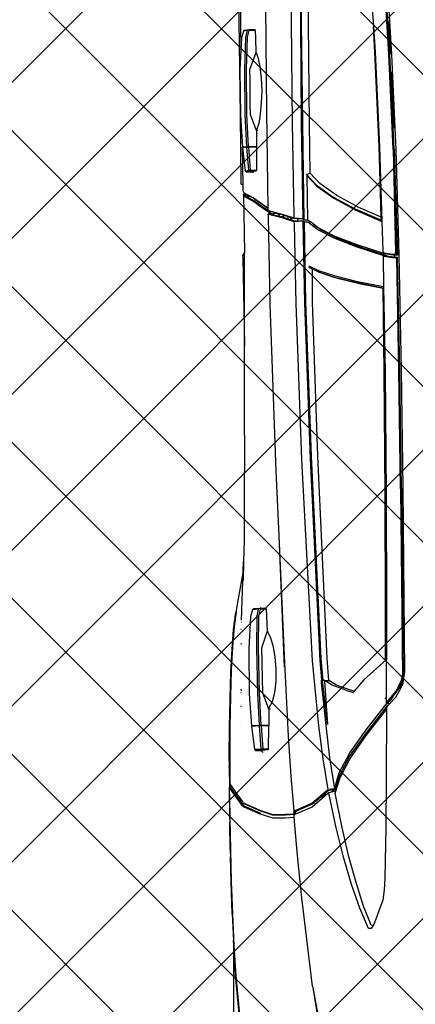
# Model space of a CAD drawing. Units: inches. Extents: x 2167 to 2589, y 1680 to 2489.
# Tile 15 of 38: x 2335 to 2353, y 1727 to 1772. Entities that reach past the tile are written whole.
import ezdxf

# ---------------------------------------------------------------- set-up
doc = ezdxf.new("R2010")
doc.units = ezdxf.units.IN
doc.header["$MEASUREMENT"] = 0
doc.layers.get('0').update_dxf_attribs({"color": 250})
doc.layers.add('C-PRKG-VEHS', color=8, linetype='Continuous', lineweight=13)
doc.layers.add('L-PVMT-PATT', color=252, linetype='Continuous', lineweight=13)
doc.layers.add('Edges', color=250, linetype='Continuous')

# ---------------------------------------------------------------- blocks, each defined once
blk = doc.blocks.new('Nissan Qashqai pl')
at = {"layer": 'Edges'}
for p, q in [((9.6953, 11.2892), (9.863, 11.2944)), ((9.6954, 11.2907), (9.8641, 11.2959)), ((9.696, 11.2932), (9.8644, 11.2982)), ((9.7669, 11.2945), (9.7832, 11.2951)), ((9.8629, 11.2925), (9.863, 11.2944)), ((9.8641, 11.2959), (9.863, 11.2944)), ((9.8638, 11.2934), (9.8641, 11.2959)), ((9.8644, 11.2982), (10.0472, 11.3018)), ((9.8681, 11.2959), (9.8678, 11.2935)), ((10.0476, 11.2996), (9.8681, 11.2959)), ((9.8681, 11.2959), (9.869, 11.2946)), ((9.869, 11.2946), (9.8689, 11.2927)), ((10.0477, 11.2982), (9.869, 11.2946)), ((10.0472, 11.3018), (10.2357, 11.3043)), ((10.2367, 11.3022), (10.0476, 11.2996)), ((10.2369, 11.3008), (10.0477, 11.2982)), ((10.2357, 11.3043), (10.53, 11.3068)), ((10.2367, 11.3022), (10.5351, 11.305)), ((10.2369, 11.3008), (10.5348, 11.3036)), ((10.4153, 11.3058), (10.2954, 11.3046)), ((10.4153, 11.3058), (10.4174, 11.3058)), ((10.4174, 11.3058), (10.4181, 11.3058)), ((10.4181, 11.3058), (10.4182, 11.3058)), ((10.4182, 11.3058), (10.53, 11.3068)), ((10.53, 11.3068), (10.5301, 11.3068)), ((10.5301, 11.3068), (10.5323, 11.3065)), ((10.5323, 11.3065), (10.5419, 11.3051)), ((10.5422, 11.3021), (10.5348, 11.3036)), ((10.5424, 11.3035), (10.5351, 11.305)), ((10.5366, 11.3048), (10.536, 11.305)), ((10.5379, 11.3052), (10.5381, 11.305)), ((10.5419, 11.3051), (10.5463, 11.3031)), ((10.5419, 11.3051), (10.5479, 11.3042)), ((10.5522, 11.2977), (10.5422, 11.3021)), ((10.5472, 11.3014), (10.5424, 11.3035)), ((10.5463, 11.3031), (10.5551, 11.2984)), ((10.5546, 11.2982), (10.5472, 11.3014)), ((10.5479, 11.3042), (10.5589, 11.2991)), ((10.5598, 11.2935), (10.5522, 11.2977)), ((10.5583, 11.296), (10.5546, 11.2982)), ((10.5551, 11.2984), (10.5583, 11.296)), ((10.5612, 11.2944), (10.5583, 11.296)), ((10.5589, 11.2991), (10.57, 11.2925)), ((10.5683, 11.2885), (10.5612, 11.2944)), ((9.5437, 11.2822), (9.4735, 11.2779)), ((9.5438, 11.2836), (9.4736, 11.2793)), ((9.4739, 11.282), (9.5443, 11.2863)), ((9.491, 11.2819), (9.5434, 11.2852)), ((9.6953, 11.2892), (9.5437, 11.2822)), ((9.6954, 11.2907), (9.5438, 11.2836)), ((9.5443, 11.2863), (9.696, 11.2932)), ((9.5717, 11.2865), (9.6618, 11.2907)), ((9.6953, 11.2892), (9.8598, 11.2925)), ((9.8652, 11.2788), (9.8516, 11.2363)), ((9.8629, 11.2925), (9.8598, 11.2925)), ((9.8605, 11.2746), (9.8626, 11.2878)), ((9.8615, 11.2754), (9.8635, 11.2886)), ((9.8626, 11.2878), (9.8627, 11.2909)), ((9.8627, 11.2909), (9.8629, 11.2925)), ((9.8627, 11.2909), (9.8637, 11.291)), ((9.8635, 11.2886), (9.8637, 11.291)), ((9.8637, 11.291), (9.8638, 11.2934)), ((9.8637, 11.291), (9.8643, 11.291)), ((9.8643, 11.291), (9.8677, 11.291)), ((9.8652, 11.2738), (9.8652, 11.2788)), ((9.8675, 11.2887), (9.8655, 11.2754)), ((9.8686, 11.2879), (9.8665, 11.2747)), ((9.8677, 11.291), (9.8675, 11.2887)), ((9.8678, 11.2935), (9.8677, 11.291)), ((9.8689, 11.2927), (9.8686, 11.2879)), ((10.2453, 11.2777), (10.4289, 11.2783)), ((10.4289, 11.2783), (10.5092, 11.2783)), ((10.5099, 11.2768), (10.5092, 11.2783)), ((10.5092, 11.2783), (10.5094, 11.2783)), ((10.5094, 11.2783), (10.51, 11.2776)), ((10.5783, 11.2783), (10.5094, 11.2783)), ((10.5764, 11.28), (10.5598, 11.2935)), ((10.5683, 11.2885), (10.573, 11.285)), ((10.575, 11.2829), (10.5683, 11.2885)), ((10.57, 11.2925), (10.5811, 11.2822)), ((10.573, 11.285), (10.5769, 11.2818)), ((10.5776, 11.2808), (10.575, 11.2829)), ((10.5783, 11.2783), (10.5764, 11.28)), ((10.5796, 11.2787), (10.5776, 11.2808)), ((10.5776, 11.2808), (10.5783, 11.2783)), ((10.5796, 11.2787), (10.5783, 11.2783)), ((10.5796, 11.2824), (10.5796, 11.2787)), ((10.6215, 11.2456), (10.5796, 11.2787)), ((10.5811, 11.2822), (10.5821, 11.2808)), ((10.5811, 11.2822), (10.5834, 11.28)), ((10.5821, 11.2808), (10.5834, 11.2793)), ((10.5825, 11.2806), (10.5834, 11.2793)), ((10.5834, 11.28), (10.5851, 11.2783)), ((10.5834, 11.2793), (10.5835, 11.2793)), ((10.5835, 11.2793), (10.584, 11.2787)), ((10.584, 11.2789), (10.584, 11.2793)), ((10.584, 11.2787), (10.584, 11.2789)), ((10.584, 11.2787), (10.6261, 11.2458)), ((10.584, 11.2787), (10.5851, 11.2783)), ((10.5843, 11.2787), (10.584, 11.2787)), ((10.5847, 11.2787), (10.5843, 11.2787)), ((10.5851, 11.2783), (10.5892, 11.2783)), ((10.6306, 11.2459), (10.5892, 11.2783)), ((10.5892, 11.2783), (10.6988, 11.2779)), ((10.6988, 11.2779), (10.7769, 11.2774)), ((9.5403, 11.26), (9.6913, 11.2674)), ((9.6912, 11.2667), (9.5404, 11.2598)), ((9.8039, 11.27), (9.6912, 11.2667)), ((9.6913, 11.2674), (9.8099, 11.2711)), ((9.8039, 11.27), (9.7884, 11.2343)), ((9.7905, 11.2283), (9.8087, 11.2702)), ((9.7925, 11.2294), (9.8107, 11.2711)), ((9.8087, 11.2702), (9.8039, 11.27)), ((9.8099, 11.2711), (9.8087, 11.2702)), ((9.8099, 11.2711), (9.8107, 11.2711)), ((9.8107, 11.2711), (9.8573, 11.2726)), ((9.8475, 11.2312), (9.8611, 11.2734)), ((9.8652, 11.2738), (9.8516, 11.2313)), ((9.8573, 11.2726), (9.8603, 11.2727)), ((9.8603, 11.2727), (9.8605, 11.2746)), ((9.8611, 11.2734), (9.8603, 11.2727)), ((9.8612, 11.2735), (9.8611, 11.2734)), ((9.8612, 11.2735), (9.8615, 11.2754)), ((9.8655, 11.2754), (9.8652, 11.2738)), ((9.8652, 11.2735), (9.8665, 11.2747)), ((9.8652, 11.2738), (9.8652, 11.2738)), ((9.8652, 11.2738), (9.8652, 11.2735)), ((9.8652, 11.2735), (9.8664, 11.2728)), ((9.8665, 11.2747), (9.8664, 11.2728)), ((9.8664, 11.2728), (9.9149, 11.2736)), ((9.9149, 11.2736), (9.9066, 11.2322)), ((9.9169, 11.2728), (9.9086, 11.2313)), ((9.9177, 11.2728), (9.9106, 11.2373)), ((9.9149, 11.2736), (10.0505, 11.276)), ((9.9177, 11.2728), (9.9169, 11.2728)), ((10.0501, 11.2747), (9.9177, 11.2728)), ((10.2453, 11.2762), (10.0501, 11.2747)), ((10.0505, 11.276), (10.2453, 11.2777)), ((10.4292, 11.2767), (10.2453, 11.2762)), ((10.5099, 11.2768), (10.4292, 11.2767)), ((10.51, 11.2776), (10.5099, 11.2768)), ((10.51, 11.2776), (10.5419, 11.2423)), ((10.5705, 11.2771), (10.5709, 11.2767)), ((10.5709, 11.2767), (10.5719, 11.2759)), ((10.7769, 11.2774), (10.858, 11.2759)), ((10.858, 11.2759), (10.8766, 11.2745)), ((10.8766, 11.2745), (10.8932, 11.2722)), ((10.8932, 11.2722), (10.932, 11.258)), ((9.471, 11.2554), (9.4997, 11.2573)), ((9.4997, 11.2573), (9.5403, 11.26)), ((9.5404, 11.2598), (9.4997, 11.2573)), ((10.933, 11.2541), (10.9026, 11.2417)), ((10.9384, 11.2497), (10.9059, 11.2355)), ((10.932, 11.258), (10.9335, 11.257)), ((10.9335, 11.257), (10.933, 11.2541)), ((10.9335, 11.257), (10.9386, 11.2537)), ((10.9386, 11.2537), (10.9384, 11.2497)), ((9.7884, 11.2343), (9.7692, 11.1989)), ((9.8338, 11.1956), (9.8475, 11.2312)), ((9.8516, 11.2363), (9.8378, 11.2007)), ((9.8516, 11.2313), (9.8378, 11.1957)), ((9.9066, 11.2322), (9.8978, 11.197)), ((9.9086, 11.2313), (9.8998, 11.196)), ((9.9106, 11.2373), (9.9018, 11.2021)), ((10.5419, 11.2423), (10.56, 11.2265)), ((10.6583, 11.2197), (10.6215, 11.2456)), ((10.6261, 11.2458), (10.6627, 11.22)), ((10.6671, 11.2203), (10.6306, 11.2459)), ((10.9026, 11.2417), (10.8653, 11.2297)), ((10.9059, 11.2355), (10.8682, 11.2226)), ((9.7713, 11.1929), (9.7905, 11.2283)), ((9.7733, 11.194), (9.7925, 11.2294)), ((10.5584, 11.2206), (10.5502, 11.1986)), ((10.56, 11.2265), (10.5584, 11.2206)), ((10.5584, 11.2136), (10.5617, 11.2251)), ((10.56, 11.2265), (10.5617, 11.2251)), ((10.69, 11.2028), (10.6583, 11.2197)), ((10.6627, 11.22), (10.6943, 11.2032)), ((10.6976, 11.2041), (10.6671, 11.2203)), ((10.8239, 11.2181), (10.7754, 11.2071)), ((10.8653, 11.2297), (10.8239, 11.2181)), ((10.8682, 11.2226), (10.8264, 11.21)), ((9.8378, 11.2007), (9.8241, 11.1736)), ((9.9018, 11.2021), (9.8931, 11.1752)), ((10.5584, 11.2136), (10.5502, 11.1916)), ((10.7155, 11.1952), (10.69, 11.2028)), ((10.6943, 11.2032), (10.7155, 11.1969)), ((10.7228, 11.1965), (10.6976, 11.2041)), ((10.7754, 11.2071), (10.7228, 11.1965)), ((10.8264, 11.21), (10.7776, 11.1982)), ((9.7692, 11.1989), (9.7499, 11.1721)), ((9.7519, 11.1661), (9.7713, 11.1929)), ((9.754, 11.1672), (9.7733, 11.194)), ((9.8201, 11.1685), (9.8338, 11.1956)), ((9.8378, 11.1957), (9.8241, 11.1686)), ((9.8978, 11.197), (9.8891, 11.1701)), ((9.8911, 11.1693), (9.8998, 11.196)), ((10.543, 11.1865), (10.5079, 11.1835)), ((10.5502, 11.1986), (10.543, 11.1865)), ((10.5502, 11.1916), (10.543, 11.1795)), ((10.543, 11.1795), (10.543, 11.1865)), ((10.5439, 11.1796), (10.613, 11.1841)), ((10.613, 11.1841), (10.547, 11.1767)), ((10.6144, 11.1813), (10.6664, 11.1875)), ((10.6664, 11.1875), (10.7155, 11.1952)), ((10.7137, 11.1846), (10.6678, 11.177)), ((10.7165, 11.1851), (10.7137, 11.1846)), ((10.7155, 11.1957), (10.7155, 11.1969)), ((10.7155, 11.1969), (10.7192, 11.1957)), ((10.7209, 11.1902), (10.7155, 11.1957)), ((10.7155, 11.1952), (10.7155, 11.1957)), ((10.7186, 11.1848), (10.7155, 11.1952)), ((10.7155, 11.1952), (10.7165, 11.1851)), ((10.7177, 11.1838), (10.7165, 11.1851)), ((10.7387, 11.1593), (10.7177, 11.1838)), ((10.7312, 11.1701), (10.7186, 11.1848)), ((10.7192, 11.1957), (10.7228, 11.1965)), ((10.7192, 11.1957), (10.7209, 11.1902)), ((10.7209, 11.1902), (10.7221, 11.1861)), ((10.7221, 11.1861), (10.7222, 11.1859)), ((10.7222, 11.186), (10.7221, 11.1861)), ((10.7247, 11.1867), (10.7222, 11.186)), ((10.7222, 11.186), (10.7222, 11.1859)), ((10.7222, 11.1859), (10.7232, 11.1848)), ((10.7222, 11.1859), (10.7224, 11.1855)), ((10.7224, 11.1855), (10.7312, 11.1701)), ((10.7232, 11.1848), (10.7228, 11.1859)), ((10.7232, 11.1848), (10.7449, 11.1598)), ((10.7776, 11.1982), (10.7247, 11.1867)), ((10.7257, 11.1853), (10.7256, 11.1854)), ((11.0357, 11.1613), (11.1598, 11.1847)), ((9.7499, 11.1721), (9.7337, 11.1566)), ((9.8241, 11.1686), (9.8119, 11.1529)), ((9.8241, 11.1736), (9.8147, 11.1616)), ((9.8147, 11.1616), (9.8201, 11.1685)), ((9.8891, 11.1701), (9.8818, 11.1551)), ((9.8911, 11.1691), (9.8867, 11.16)), ((9.8931, 11.1751), (9.8911, 11.1693)), ((9.8911, 11.1693), (9.8911, 11.1691)), ((9.8931, 11.1751), (9.8931, 11.1752)), ((10.1849, 11.1687), (9.9393, 11.1602)), ((10.5079, 11.1835), (10.1849, 11.1687)), ((10.5079, 11.1739), (10.1849, 11.1585)), ((10.1894, 11.1563), (10.5109, 11.1721)), ((10.543, 11.1771), (10.5079, 11.1739)), ((10.5109, 11.1721), (10.5417, 11.1748)), ((10.6152, 11.1702), (10.5113, 11.1603)), ((10.543, 11.1771), (10.5417, 11.1748)), ((10.5417, 11.1748), (10.5427, 11.1739)), ((10.5436, 11.1754), (10.5427, 11.1739)), ((10.5427, 11.1739), (10.5458, 11.1742)), ((10.5439, 11.1796), (10.543, 11.1795)), ((10.543, 11.1795), (10.543, 11.1771)), ((10.544, 11.1763), (10.543, 11.1771)), ((10.544, 11.1763), (10.5436, 11.1754)), ((10.547, 11.1767), (10.544, 11.1763)), ((10.5458, 11.1742), (10.6144, 11.1813)), ((10.6678, 11.177), (10.6152, 11.1702)), ((10.7397, 11.1602), (10.7312, 11.1701)), ((11.0492, 11.1635), (11.1336, 11.1772)), ((9.4936, 11.1538), (9.3225, 11.1531)), ((9.6552, 11.1554), (9.4936, 11.1538)), ((9.7337, 11.1566), (9.6552, 11.1554)), ((9.7357, 11.1507), (9.7337, 11.1566)), ((9.7357, 11.1507), (9.7519, 11.1661)), ((9.7378, 11.1517), (9.754, 11.1672)), ((9.8078, 11.1528), (9.7378, 11.1517)), ((9.8078, 11.1528), (9.8119, 11.1579)), ((9.8078, 11.1471), (9.8078, 11.1528)), ((9.8147, 11.1616), (9.8119, 11.1579)), ((9.8119, 11.1579), (9.8119, 11.1529)), ((9.8119, 11.1529), (9.8119, 11.1472)), ((9.8147, 11.1616), (9.8147, 11.1616)), ((9.8867, 11.16), (9.8838, 11.1541)), ((9.9393, 11.1602), (9.8867, 11.16)), ((10.1849, 11.1585), (9.9393, 11.1497)), ((9.9411, 11.1475), (10.1894, 11.1563)), ((10.5113, 11.1603), (10.19, 11.1433)), ((10.7501, 11.1327), (10.7387, 11.1593)), ((10.7507, 11.1344), (10.7397, 11.1602)), ((10.7449, 11.1598), (10.7563, 11.1333)), ((11.0304, 11.1603), (10.8896, 11.1434)), ((11.0304, 11.1603), (11.0357, 11.1613)), ((11.0357, 11.1613), (11.0491, 11.1635)), ((11.0492, 11.1635), (11.0491, 11.1635)), ((9.3198, 11.1403), (9.4922, 11.1409)), ((9.4936, 11.1428), (9.3225, 11.1421)), ((9.4922, 11.1409), (9.654, 11.1423)), ((9.6552, 11.1445), (9.4936, 11.1428)), ((9.654, 11.1423), (9.8061, 11.1447)), ((9.8078, 11.1471), (9.6552, 11.1445)), ((9.7357, 11.1507), (9.7378, 11.1517)), ((9.8061, 11.1447), (9.8051, 11.1309)), ((9.8055, 11.1298), (9.8058, 11.1369)), ((9.8058, 11.1369), (9.8061, 11.1447)), ((9.8098, 11.1369), (9.8058, 11.1369)), ((9.8061, 11.1447), (9.8078, 11.1471)), ((9.8098, 11.1369), (9.8096, 11.13)), ((9.8101, 11.1449), (9.8098, 11.1369)), ((9.8101, 11.1449), (9.9411, 11.1475)), ((9.8119, 11.1472), (9.8101, 11.1449)), ((9.8101, 11.1449), (9.8112, 11.1311)), ((9.9393, 11.1497), (9.8119, 11.1472)), ((10.19, 11.1433), (9.9414, 11.1341)), ((10.8218, 11.1365), (10.7615, 11.1311)), ((10.8896, 11.1434), (10.8218, 11.1365)), ((9.4919, 11.1269), (9.3194, 11.1262)), ((9.6538, 11.1284), (9.4919, 11.1269)), ((9.802, 11.1309), (9.6538, 11.1284)), ((9.7992, 11.1133), (9.8044, 11.129)), ((9.803, 11.1212), (9.8014, 11.1176)), ((9.8014, 11.1176), (9.8026, 11.1212)), ((9.8051, 11.1309), (9.802, 11.1309)), ((9.8026, 11.1212), (9.8041, 11.1256)), ((9.803, 11.1212), (9.8026, 11.1212)), ((9.8067, 11.1213), (9.803, 11.1212)), ((9.8041, 11.1256), (9.8045, 11.1268)), ((9.8041, 11.1256), (9.8081, 11.1256)), ((9.8044, 11.129), (9.8051, 11.1309)), ((9.8067, 11.1213), (9.8044, 11.1142)), ((9.8045, 11.1268), (9.8046, 11.1271)), ((9.8045, 11.1268), (9.8085, 11.1268)), ((9.8046, 11.1271), (9.8055, 11.1298)), ((9.8086, 11.1271), (9.8046, 11.1271)), ((9.8106, 11.1292), (9.8054, 11.1135)), ((9.8081, 11.1256), (9.8067, 11.1213)), ((9.8085, 11.1268), (9.8081, 11.1256)), ((9.8086, 11.1271), (9.8085, 11.1268)), ((9.8096, 11.13), (9.8086, 11.1271)), ((9.8112, 11.1311), (9.8106, 11.1292)), ((9.8143, 11.1312), (9.8112, 11.1311)), ((9.9414, 11.1341), (9.8143, 11.1312)), ((10.5147, 11.1156), (10.6318, 11.1213)), ((10.6318, 11.1213), (10.6955, 11.1257)), ((10.6955, 11.1257), (10.7509, 11.1302)), ((10.7507, 11.1309), (10.7501, 11.1327)), ((10.7511, 11.1335), (10.7507, 11.1344)), ((10.7507, 11.1344), (10.7524, 11.1335)), ((10.751, 11.131), (10.7507, 11.1309)), ((10.7509, 11.1302), (10.7507, 11.1309)), ((10.7522, 11.1311), (10.7509, 11.1302)), ((10.7516, 11.131), (10.7509, 11.1302)), ((10.7519, 11.1314), (10.7511, 11.1335)), ((10.7519, 11.1314), (10.7516, 11.131)), ((10.7522, 11.1311), (10.7516, 11.131)), ((10.7526, 11.1318), (10.7519, 11.1314)), ((10.7553, 11.1307), (10.7522, 11.1311)), ((10.7524, 11.1335), (10.7526, 11.1318)), ((10.7524, 11.1335), (10.7556, 11.1319)), ((10.7532, 11.1321), (10.7526, 11.1318)), ((10.7526, 11.1318), (10.7526, 11.1314)), ((10.7556, 11.1319), (10.7532, 11.1321)), ((10.7563, 11.1169), (10.7553, 11.1307)), ((10.7556, 11.1319), (10.7561, 11.1317)), ((10.7563, 11.1319), (10.7561, 11.1319)), ((10.7563, 11.1315), (10.7561, 11.1317)), ((10.7561, 11.1317), (10.7563, 11.1317)), ((10.7563, 11.1333), (10.7569, 11.1317)), ((10.7563, 11.1317), (10.7563, 11.1319)), ((10.7563, 11.1317), (10.7569, 11.1317)), ((10.7569, 11.1316), (10.7563, 11.1317)), ((10.7563, 11.1315), (10.7563, 11.1317)), ((10.7572, 11.1178), (10.7563, 11.1315)), ((10.7573, 11.1307), (10.7563, 11.1315)), ((10.7569, 11.1317), (10.7569, 11.1316)), ((10.7569, 11.1316), (10.7573, 11.1307)), ((10.7604, 11.131), (10.7573, 11.1307)), ((10.7615, 11.1311), (10.7604, 11.131)), ((10.7615, 11.1311), (10.7623, 11.1173)), ((9.7937, 11.0918), (9.7992, 11.1133)), ((9.7987, 11.1053), (9.7977, 11.1033)), ((9.7978, 11.1044), (9.7987, 11.108)), ((9.7987, 11.1053), (9.7978, 11.1044)), ((9.7987, 11.108), (9.8002, 11.1141)), ((9.7992, 11.1065), (9.7987, 11.108)), ((9.7992, 11.1065), (9.7987, 11.1053)), ((9.8027, 11.1078), (9.7992, 11.1065)), ((9.8054, 11.1135), (9.7999, 11.0919)), ((9.8002, 11.1141), (9.8008, 11.1157)), ((9.8027, 11.1078), (9.8003, 11.0983)), ((9.8008, 11.1157), (9.8014, 11.1176)), ((9.8014, 11.1139), (9.8008, 11.1157)), ((9.8043, 11.1139), (9.8014, 11.1139)), ((9.8031, 11.1093), (9.8014, 11.1139)), ((9.8031, 11.1093), (9.8027, 11.1078)), ((9.8043, 11.1139), (9.8031, 11.1093)), ((9.8044, 11.1142), (9.8043, 11.1139)), ((10.2081, 11.1017), (10.312, 11.1064)), ((10.312, 11.1064), (10.5147, 11.1156)), ((10.312, 11.1064), (10.5214, 11.1149)), ((10.7565, 11.0969), (10.7563, 11.1169)), ((10.7575, 11.0979), (10.7572, 11.1178)), ((10.7623, 11.1173), (10.7626, 11.0974)), ((9.7965, 11.0915), (9.7894, 11.0806)), ((9.7931, 11.089), (9.7934, 11.0906)), ((9.7933, 11.0892), (9.7941, 11.0901)), ((9.7934, 11.0906), (9.7937, 11.0918)), ((9.7934, 11.0906), (9.7938, 11.0904)), ((9.7941, 11.0901), (9.7943, 11.0907)), ((9.7964, 11.0988), (9.7943, 11.0907)), ((9.7955, 11.0925), (9.7943, 11.0907)), ((9.7963, 11.0918), (9.7955, 11.0925)), ((9.7992, 11.0966), (9.7963, 11.0918)), ((9.7963, 11.0918), (9.7963, 11.0918)), ((9.7964, 11.0917), (9.7963, 11.0918)), ((9.7964, 11.0988), (9.7973, 11.1023)), ((9.7964, 11.0988), (9.7992, 11.0966)), ((9.7964, 11.0917), (9.7996, 11.0966)), ((9.7964, 11.0917), (9.7964, 11.0917)), ((9.7967, 11.0915), (9.7964, 11.0917)), ((9.7965, 11.0915), (9.7967, 11.0915)), ((9.7983, 11.0901), (9.7965, 11.0915)), ((9.7967, 11.0915), (9.7986, 11.0916)), ((9.7977, 11.0907), (9.7967, 11.0915)), ((9.7973, 11.1023), (9.7977, 11.1042)), ((9.7977, 11.1033), (9.7973, 11.1023)), ((9.7973, 11.1023), (9.7977, 11.1011)), ((9.7977, 11.1042), (9.7978, 11.1044)), ((9.7977, 11.1042), (9.7977, 11.1033)), ((9.7977, 11.1011), (9.7977, 11.0998)), ((9.7977, 11.1011), (9.7985, 11.099)), ((9.7977, 11.0998), (9.7985, 11.099)), ((9.7982, 11.0902), (9.7977, 11.0907)), ((9.7986, 11.0916), (9.7982, 11.0902)), ((9.7983, 11.0901), (9.7982, 11.0902)), ((9.7986, 11.0898), (9.7983, 11.0901)), ((9.7985, 11.099), (9.7989, 11.098)), ((9.7988, 11.0925), (9.7986, 11.0916)), ((9.7986, 11.0898), (9.7993, 11.0891)), ((9.7998, 11.0964), (9.7988, 11.0925)), ((9.7989, 11.098), (9.7998, 11.0976)), ((9.7998, 11.0976), (9.7992, 11.0966)), ((9.7999, 11.0919), (9.7993, 11.0891)), ((9.8002, 11.098), (9.7996, 11.0966)), ((9.8001, 11.0974), (9.7996, 11.0966)), ((9.7996, 11.0966), (9.7998, 11.0964)), ((9.8003, 11.0983), (9.7998, 11.0976)), ((9.8001, 11.0974), (9.7998, 11.0964)), ((9.8002, 11.098), (9.8001, 11.0974)), ((9.8003, 11.0983), (9.8002, 11.098)), ((9.8024, 11.0892), (9.9426, 11.0923)), ((9.9426, 11.0923), (10.2081, 11.1017)), ((10.4653, 11.0881), (10.4652, 11.0897)), ((10.4653, 11.0881), (10.4732, 11.0925)), ((10.4732, 11.0925), (10.4871, 11.0967)), ((10.4871, 11.0967), (10.5048, 11.1002)), ((10.5048, 11.1002), (10.5246, 11.1019)), ((10.5246, 11.1019), (10.5445, 11.1017)), ((10.5445, 11.1017), (10.5625, 11.0996)), ((10.5625, 11.0996), (10.5769, 11.0957)), ((10.5867, 11.0897), (10.563, 11.0809)), ((10.5769, 11.0957), (10.5863, 11.0904)), ((10.5863, 11.0904), (10.5867, 11.0897)), ((10.5885, 11.0904), (10.5867, 11.0897)), ((10.5885, 11.0931), (10.5885, 11.0904)), ((10.5885, 11.0904), (10.6141, 11.0905)), ((10.6141, 11.0905), (10.615, 11.0905)), ((10.6142, 11.0782), (10.6141, 11.0905)), ((10.6517, 11.0902), (10.615, 11.0905)), ((10.615, 11.0905), (10.6151, 11.0782)), ((10.6518, 11.0808), (10.6517, 11.0902)), ((10.6517, 11.0902), (10.6535, 11.0895)), ((10.6535, 11.0895), (10.6543, 11.0786)), ((10.6535, 11.0895), (10.6536, 11.0803)), ((10.7497, 11.0763), (10.7565, 11.0969)), ((10.7507, 11.0773), (10.7575, 11.0979)), ((10.7626, 11.0974), (10.7559, 11.0767)), ((9.4673, 11.0852), (9.6358, 11.0866)), ((9.5503, 11.0736), (9.5641, 11.076)), ((9.5641, 11.076), (9.5818, 11.0782)), ((9.5818, 11.0782), (9.6016, 11.0791)), ((9.6016, 11.0791), (9.6215, 11.0782)), ((9.6215, 11.0782), (9.6395, 11.0766)), ((9.6358, 11.0866), (9.7887, 11.0889)), ((9.6395, 11.0766), (9.654, 11.0744)), ((9.654, 11.0744), (9.6633, 11.0715)), ((9.7728, 11.066), (9.7832, 11.0805)), ((9.7738, 11.067), (9.7842, 11.0814)), ((9.7883, 11.0815), (9.7778, 11.0671)), ((9.7894, 11.0806), (9.7788, 11.0661)), ((9.7832, 11.0805), (9.7887, 11.0889)), ((9.7842, 11.0814), (9.7891, 11.0889)), ((9.7933, 11.0892), (9.7883, 11.0815)), ((9.7887, 11.0889), (9.7891, 11.0889)), ((9.7891, 11.0889), (9.79, 11.0889)), ((9.79, 11.0889), (9.7931, 11.089)), ((9.7931, 11.089), (9.7933, 11.0892)), ((9.7993, 11.0891), (9.8024, 11.0892)), ((10.4263, 11.0777), (10.4274, 11.0767)), ((10.4274, 11.0767), (10.4275, 11.0856)), ((10.4274, 11.0762), (10.4274, 11.0767)), ((10.4282, 11.0666), (10.4274, 11.0762)), ((10.4275, 11.0856), (10.4293, 11.0863)), ((10.4293, 11.0863), (10.4291, 11.0765)), ((10.4291, 11.0765), (10.4398, 11.0741)), ((10.4398, 11.0718), (10.4291, 11.0741)), ((10.4291, 11.0741), (10.4299, 11.0644)), ((10.4293, 11.0863), (10.4398, 11.0868)), ((10.4398, 11.0868), (10.4653, 11.0878)), ((10.4398, 11.0741), (10.4909, 11.0734)), ((10.4653, 11.0877), (10.4653, 11.0881)), ((10.4653, 11.0878), (10.4653, 11.0881)), ((10.4653, 11.0881), (10.4653, 11.0881)), ((10.4653, 11.0877), (10.4653, 11.0878)), ((10.4908, 11.0793), (10.4653, 11.0877)), ((10.563, 11.0809), (10.4908, 11.0793)), ((10.4909, 11.0734), (10.563, 11.075)), ((10.563, 11.075), (10.6142, 11.0779)), ((10.6142, 11.0756), (10.5631, 11.0727)), ((10.6142, 11.0779), (10.6142, 11.0782)), ((10.6142, 11.0765), (10.6142, 11.0779)), ((10.615, 11.0765), (10.6142, 11.0765)), ((10.6142, 11.0756), (10.6142, 11.0765)), ((10.615, 11.0639), (10.6142, 11.0756)), ((10.6151, 11.0765), (10.615, 11.0765)), ((10.615, 11.0765), (10.6151, 11.0639)), ((10.6151, 11.078), (10.6518, 11.0808)), ((10.6518, 11.0784), (10.6151, 11.0756)), ((10.6151, 11.0782), (10.6151, 11.078)), ((10.6151, 11.078), (10.6151, 11.0765)), ((10.6151, 11.0765), (10.6151, 11.0756)), ((10.6151, 11.0756), (10.616, 11.0629)), ((10.6518, 11.0784), (10.6518, 11.0808)), ((10.6518, 11.0808), (10.6536, 11.0803)), ((10.6536, 11.0803), (10.6518, 11.0784)), ((10.6526, 11.0674), (10.6518, 11.0784)), ((10.6536, 11.0803), (10.6537, 11.0783)), ((10.6543, 11.0786), (10.6537, 11.0783)), ((10.6537, 11.0783), (10.6543, 11.0693)), ((10.6578, 11.0814), (10.6543, 11.0786)), ((10.6543, 11.0693), (10.6543, 11.0786)), ((10.7385, 11.051), (10.7497, 11.0763)), ((10.7396, 11.0519), (10.7507, 11.0773)), ((10.7549, 11.0776), (10.743, 11.0503)), ((10.7559, 11.0767), (10.7448, 11.0511)), ((9.5037, 11.0635), (9.5045, 11.0628)), ((9.5044, 11.0586), (9.5045, 11.0628)), ((9.5052, 11.0524), (9.5044, 11.0586)), ((9.5045, 11.0683), (9.5063, 11.0687)), ((9.5045, 11.0628), (9.5045, 11.0683)), ((9.5063, 11.0687), (9.5061, 11.0586)), ((9.5061, 11.0586), (9.5167, 11.0559)), ((9.5063, 11.0687), (9.5168, 11.0691)), ((9.5168, 11.0691), (9.5423, 11.0696)), ((9.5422, 11.0706), (9.5422, 11.0716)), ((9.5422, 11.0706), (9.5424, 11.0707)), ((9.5423, 11.0696), (9.5422, 11.0706)), ((9.5426, 11.0695), (9.5423, 11.0696)), ((9.5424, 11.0707), (9.5503, 11.0736)), ((9.5426, 11.0695), (9.5424, 11.0707)), ((9.5667, 11.0609), (9.5426, 11.0695)), ((9.5678, 11.0604), (9.5667, 11.0609)), ((9.5846, 11.0606), (9.5678, 11.0604)), ((9.6236, 11.0609), (9.5846, 11.0606)), ((9.64, 11.0611), (9.6236, 11.0609)), ((9.6413, 11.0616), (9.64, 11.0611)), ((9.6645, 11.0705), (9.6413, 11.0616)), ((9.6633, 11.0715), (9.6645, 11.0705)), ((9.6655, 11.0708), (9.6645, 11.0705)), ((9.6655, 11.0728), (9.6655, 11.0708)), ((9.6655, 11.0708), (9.6911, 11.0709)), ((9.6911, 11.0709), (9.692, 11.0709)), ((9.6911, 11.0645), (9.6911, 11.0709)), ((9.6912, 11.0631), (9.6911, 11.0645)), ((9.692, 11.0631), (9.6912, 11.0631)), ((9.6912, 11.0577), (9.6912, 11.0631)), ((9.692, 11.0709), (9.692, 11.0645)), ((9.692, 11.0709), (9.7287, 11.0708)), ((9.692, 11.0645), (9.692, 11.0631)), ((9.692, 11.0631), (9.6921, 11.0578)), ((9.6921, 11.0578), (9.7288, 11.0609)), ((9.7288, 11.0588), (9.6922, 11.0556)), ((9.7287, 11.0708), (9.7305, 11.0704)), ((9.7288, 11.0609), (9.7287, 11.0708)), ((9.7288, 11.0588), (9.7288, 11.0609)), ((9.7288, 11.0609), (9.7306, 11.0607)), ((9.7306, 11.0607), (9.7288, 11.0588)), ((9.7296, 11.0527), (9.7288, 11.0588)), ((9.7305, 11.0704), (9.7313, 11.0644)), ((9.7305, 11.0704), (9.7306, 11.0607)), ((9.7306, 11.0607), (9.7314, 11.0547)), ((9.733, 11.066), (9.7313, 11.0644)), ((9.7314, 11.0547), (9.7313, 11.0644)), ((9.7674, 11.0557), (9.7728, 11.066)), ((9.7684, 11.0567), (9.7717, 11.0631)), ((9.7717, 11.0631), (9.7707, 11.0593)), ((9.7707, 11.0593), (9.7709, 11.0549)), ((9.7717, 11.0631), (9.7738, 11.067)), ((9.7778, 11.0671), (9.7724, 11.0568)), ((9.7788, 11.0661), (9.7734, 11.0558)), ((10.4282, 11.0666), (10.4299, 11.0644)), ((10.4299, 11.0644), (10.4406, 11.0612)), ((10.4909, 11.0711), (10.4398, 11.0718)), ((10.4406, 11.0612), (10.4919, 11.0584)), ((10.5631, 11.0727), (10.4909, 11.0711)), ((10.4919, 11.0584), (10.564, 11.0591)), ((10.564, 11.0591), (10.6151, 11.0628)), ((10.6151, 11.0639), (10.615, 11.0639)), ((10.6151, 11.0628), (10.615, 11.0639)), ((10.6151, 11.0639), (10.6151, 11.0628)), ((10.616, 11.0629), (10.6526, 11.0674)), ((10.6526, 11.0674), (10.6543, 11.0693)), ((9.2517, 11.0411), (9.5372, 11.0459)), ((9.641, 11.045), (9.351, 11.0411)), ((9.5052, 11.0524), (9.5069, 11.0501)), ((9.5168, 11.0537), (9.5061, 11.0564)), ((9.5061, 11.0564), (9.5069, 11.0501)), ((9.5069, 11.0501), (9.5176, 11.0469)), ((9.5167, 11.0559), (9.5679, 11.0543)), ((9.5679, 11.0521), (9.5168, 11.0537)), ((9.5176, 11.0469), (9.5372, 11.0459)), ((9.5372, 11.0459), (9.5689, 11.0442)), ((9.5679, 11.0543), (9.64, 11.0549)), ((9.6401, 11.0528), (9.5679, 11.0521)), ((9.5689, 11.0442), (9.641, 11.045)), ((9.64, 11.0549), (9.6912, 11.0577)), ((9.6913, 11.0556), (9.6401, 11.0528)), ((9.641, 11.045), (9.6921, 11.0485)), ((9.7466, 11.0464), (9.641, 11.045)), ((9.6913, 11.0556), (9.6912, 11.0577)), ((9.692, 11.0499), (9.6913, 11.0556)), ((9.6922, 11.0499), (9.692, 11.0499)), ((9.6921, 11.0485), (9.692, 11.0499)), ((9.6922, 11.0556), (9.6921, 11.0578)), ((9.6922, 11.0499), (9.6921, 11.0485)), ((9.7526, 11.0495), (9.6921, 11.0485)), ((9.6922, 11.0556), (9.693, 11.0486)), ((9.6922, 11.0556), (9.6922, 11.0499)), ((9.693, 11.0486), (9.7296, 11.0527)), ((9.7296, 11.0527), (9.7314, 11.0547)), ((9.7511, 11.0463), (9.7466, 11.0464)), ((9.7526, 11.0495), (9.7511, 11.0463)), ((9.7623, 11.0497), (9.7526, 11.0495)), ((9.7623, 11.0497), (9.7643, 11.0504)), ((9.7643, 11.0504), (9.7652, 11.0514)), ((9.7643, 11.0504), (9.7648, 11.0513)), ((9.7648, 11.0513), (9.7664, 11.054)), ((9.7648, 11.0513), (9.7648, 11.0513)), ((9.7652, 11.0514), (9.7665, 11.0535)), ((9.7664, 11.054), (9.7674, 11.0557)), ((9.7665, 11.0537), (9.7664, 11.054)), ((9.7665, 11.0535), (9.7676, 11.0553)), ((9.7667, 11.0508), (9.7665, 11.0535)), ((9.7676, 11.0511), (9.7667, 11.0508)), ((9.7677, 11.0498), (9.7667, 11.0508)), ((9.7673, 11.0545), (9.7676, 11.0553)), ((9.7673, 11.0543), (9.7673, 11.0545)), ((9.7676, 11.0511), (9.7673, 11.0543)), ((9.7676, 11.0553), (9.7684, 11.0567)), ((9.7676, 11.0555), (9.7678, 11.056)), ((9.769, 11.0516), (9.7676, 11.0511)), ((9.7677, 11.0498), (9.8598, 11.0514)), ((9.77, 11.0506), (9.7677, 11.0498)), ((9.7677, 11.0498), (9.7677, 11.0498)), ((9.7712, 11.055), (9.769, 11.0516)), ((9.7734, 11.0558), (9.77, 11.0506)), ((9.7709, 11.0549), (9.7712, 11.055)), ((9.7724, 11.0568), (9.7712, 11.055)), ((9.8598, 11.0514), (9.8614, 11.0504)), ((9.8643, 11.0514), (9.8598, 11.0514)), ((9.8614, 11.0504), (9.8647, 11.0485)), ((10.0085, 11.0519), (9.8643, 11.0514)), ((9.8647, 11.0485), (9.869, 11.0488)), ((9.869, 11.0488), (10.0085, 11.0519)), ((10.0124, 11.0519), (10.0085, 11.0519)), ((10.1513, 11.0517), (10.0124, 11.0519)), ((10.1513, 11.0517), (10.2677, 11.0512)), ((10.2677, 11.0512), (10.3189, 11.0511)), ((10.3189, 11.0511), (10.3537, 11.0503)), ((10.3537, 11.0503), (10.3832, 11.0496)), ((10.3679, 11.0497), (10.3537, 11.0503)), ((10.3679, 11.0497), (10.4275, 11.0391)), ((10.4468, 11.0466), (10.3679, 11.0497)), ((10.4502, 11.0466), (10.4503, 11.0465)), ((10.4613, 11.0464), (10.4603, 11.0465)), ((10.4838, 11.0465), (10.4852, 11.046)), ((10.5565, 11.0456), (10.5591, 11.0464)), ((10.5615, 11.0464), (10.5617, 11.0457)), ((10.583, 11.0457), (10.5835, 11.0461)), ((10.5836, 11.0461), (10.5832, 11.0457)), ((10.5847, 11.0461), (10.5841, 11.0457)), ((10.5873, 11.0461), (10.5873, 11.0461)), ((10.6087, 11.0458), (10.6087, 11.0458)), ((10.7087, 11.0289), (10.7363, 11.0483)), ((10.7424, 11.0499), (10.7125, 11.0285)), ((10.7429, 11.0485), (10.7148, 11.0284)), ((10.7363, 11.0483), (10.7376, 11.0492)), ((10.7387, 11.0502), (10.7376, 11.0492)), ((10.7376, 11.0492), (10.7378, 11.0495)), ((10.7378, 11.0495), (10.7385, 11.051)), ((10.7378, 11.0495), (10.7379, 11.0496)), ((10.7387, 11.0502), (10.7396, 11.0519)), ((10.7424, 11.0499), (10.743, 11.0503)), ((10.7429, 11.0488), (10.7432, 11.0488)), ((10.7432, 11.0488), (10.7429, 11.0485)), ((10.744, 11.0494), (10.7432, 11.0488)), ((10.7448, 11.0511), (10.744, 11.0494)), ((11.0798, 11.0434), (11.0576, 11.0416)), ((11.059, 11.0419), (11.0768, 11.0434)), ((10.4275, 11.0391), (10.4304, 11.0385)), ((10.4304, 11.0385), (10.4339, 11.0381)), ((10.4345, 11.0379), (10.4339, 11.0381)), ((10.4339, 11.0381), (10.4573, 11.0349)), ((10.4613, 11.0343), (10.4345, 11.0379)), ((10.4573, 11.0349), (10.4889, 11.0323)), ((10.4926, 11.0317), (10.4613, 11.0343)), ((10.4889, 11.0323), (10.526, 11.0304)), ((10.5294, 11.0298), (10.4926, 11.0317)), ((10.526, 11.0304), (10.569, 11.0291)), ((10.5719, 11.0285), (10.5294, 11.0298)), ((10.569, 11.0291), (10.5919, 11.0287)), ((10.6176, 11.0277), (10.5719, 11.0285)), ((10.5919, 11.0287), (10.5936, 11.0286)), ((10.5936, 11.0286), (10.6151, 11.0283)), ((10.6151, 11.0283), (10.6644, 11.028)), ((10.6651, 11.0274), (10.6176, 11.0277)), ((10.6644, 11.028), (10.7078, 11.0282)), ((10.677, 11.0275), (10.6651, 11.0274)), ((10.7082, 11.0285), (10.6729, 11.0284)), ((10.68, 11.0274), (10.677, 11.0275)), ((10.6809, 11.0274), (10.68, 11.0274)), ((10.6809, 11.0274), (10.7128, 11.0275)), ((10.7078, 11.0282), (10.7083, 11.0285)), ((10.7082, 11.0285), (10.7078, 11.0282)), ((10.7085, 11.0289), (10.7082, 11.0285)), ((10.7083, 11.0285), (10.7082, 11.0285)), ((10.7083, 11.0285), (10.7087, 11.0289)), ((10.7125, 11.0285), (10.7083, 11.0285)), ((10.7146, 11.0286), (10.7125, 11.0285)), ((10.7125, 11.0285), (10.7139, 11.0278)), ((10.7134, 11.0275), (10.7128, 11.0275)), ((10.7625, 11.0281), (10.7134, 11.0275)), ((10.724, 11.0275), (10.7134, 11.0275)), ((10.7148, 11.0284), (10.7139, 11.0278)), ((10.7628, 11.0283), (10.7139, 11.0278)), ((10.724, 11.0275), (10.7685, 11.0281)), ((10.7628, 11.0281), (10.7625, 11.0281)), ((10.7628, 11.0283), (10.8131, 11.0292)), ((10.7628, 11.0281), (10.8131, 11.029)), ((10.7688, 11.0281), (10.7685, 11.0281)), ((10.8131, 11.029), (10.7688, 11.0281)), ((10.8131, 11.0292), (10.8644, 11.0306)), ((10.8132, 11.029), (10.8131, 11.029)), ((10.8132, 11.029), (10.8139, 11.029)), ((10.8142, 11.029), (10.8139, 11.029)), ((10.8142, 11.029), (10.8241, 11.0293)), ((10.8142, 11.029), (10.8142, 11.029)), ((10.8242, 11.0293), (10.8241, 11.0293)), ((10.8246, 11.0293), (10.8242, 11.0293)), ((10.8642, 11.0304), (10.8246, 11.0293)), ((10.9152, 11.0321), (10.8642, 11.0304)), ((10.8642, 11.0305), (10.8759, 11.031)), ((10.8644, 11.0306), (10.8759, 11.031)), ((10.8759, 11.031), (10.9158, 11.0324)), ((10.9152, 11.0321), (10.9577, 11.0341)), ((10.9158, 11.0324), (10.9657, 11.0347)), ((10.9649, 11.0344), (10.9577, 11.0341)), ((10.9577, 11.0341), (11.1283, 11.0341)), ((11.0127, 11.0375), (10.9649, 11.0344)), ((10.9657, 11.0347), (11.0138, 11.0377)), ((11.0576, 11.0416), (11.0127, 11.0375)), ((11.0138, 11.0377), (11.059, 11.0419))]:
    blk.add_line(p, q, dxfattribs=at)
blk = doc.blocks.new('car')
blk.add_blockref('Nissan Qashqai pl', (-9.7433, -11.9151))
blk = doc.blocks.new('carr')
blk.add_blockref('car', (0.5124, -0.007))

msp = doc.modelspace()

# ---------------------------------------------------------------- hatches: boundary and pattern name
at = {"layer": 'L-PVMT-PATT'}
h = msp.add_hatch(dxfattribs=at)
h.set_pattern_fill('ANSI37', color=256, scale=40)
h.paths.add_polyline_path([(2417.548, 1783.695), (2417.548, 1846.042), (2239.361, 1846.042), (2239.361, 1687.695), (2369.843, 1687.695), (2369.843, 1696.695), (2375.607, 1696.695), (2416.107, 1696.695), (2417.548, 1696.695)])

# ---------------------------------------------------------------- block references
at = {"layer": 'C-PRKG-VEHS', "xscale": 28.42784210623918, "yscale": 28.42784210623918, "zscale": 28.42784210623918, "rotation": 270}
msp.add_blockref('carr', (2369.852, 1779.037), dxfattribs=at)

doc.saveas('drawing.dxf')
